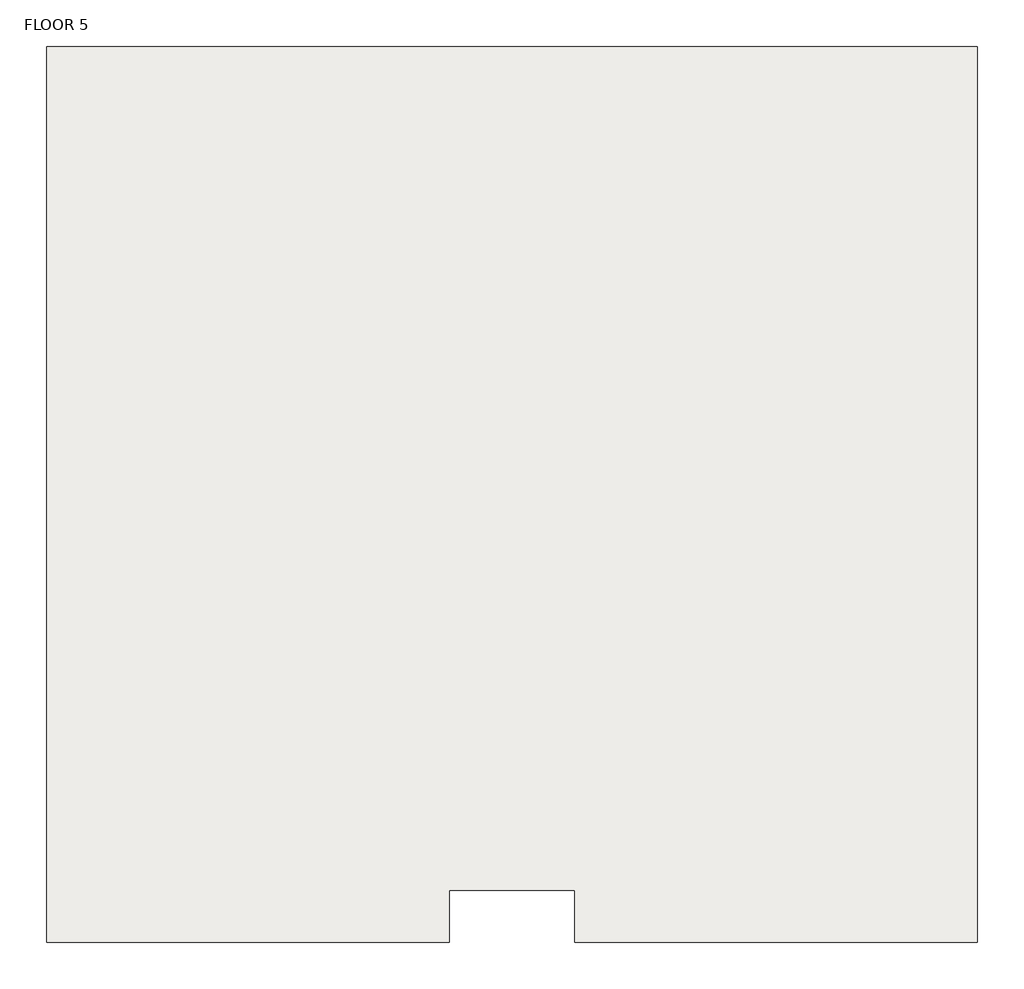
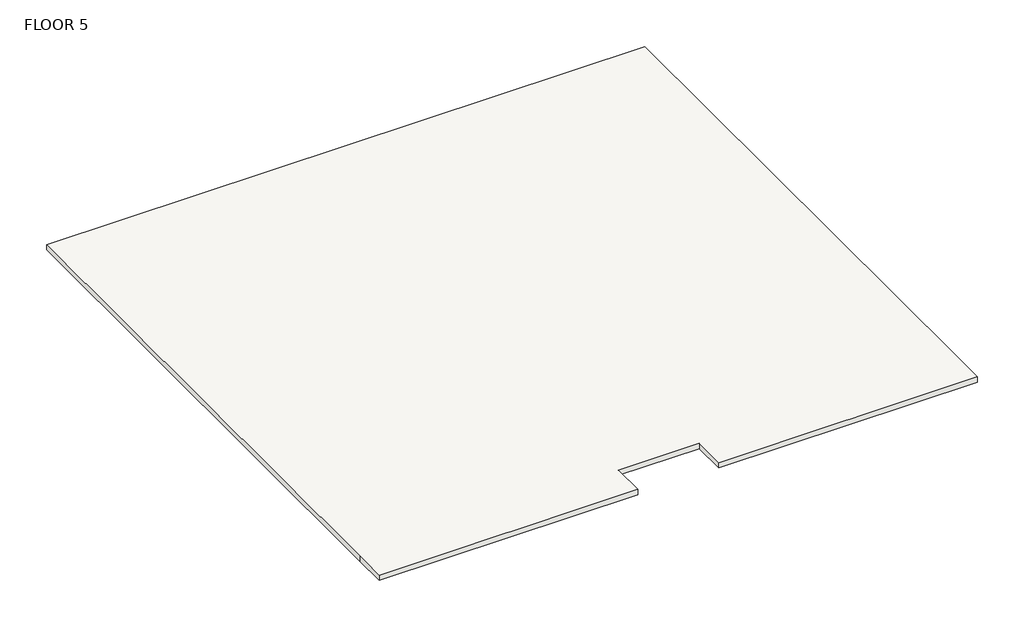
# One storey: 1 roof.
"""IFC4 building model written with IfcOpenShell, lengths in millimetres."""

from ifc_helpers import new_model, si_unit, frame, origin, place, context, project, spatial, polyline, outline, extrude, element, save

model = new_model("IFC4")

# Units and contexts
model_context = context("Model", 3, world=origin())
ifc_project = project(units=[si_unit("LENGTHUNIT", "METRE", prefix="MILLI")], contexts=[model_context])

# Site, building, storey
site = spatial("IfcSite", under=ifc_project)
building = spatial("IfcBuilding", under=site)
storey = spatial("IfcBuildingStorey", under=building, Name="FLOOR 5", Elevation=9391.9725604)

# Roof
placement = place(None, origin())
element("IfcRoof", 1, ObjectType="ROOFING 6\"", at=placement, inside=storey, context=model_context, shape_type="SweptSolid", body=[
    extrude(outline(polyline([(-3159.4137331, -7822.4593836), (-5369.2137331, -7822.4593836), (-5369.2137331, -8736.8593836), (-12430.4137331, -8736.8593836), (-12430.4137331, -7822.4593836), (-12430.4137331, 6987.3281164), (3901.7862669, 6987.3281164), (3901.7862669, -7822.4593836), (3901.7862669, -8736.8593836), (-3159.4137331, -8736.8593836), (-3159.4137331, -7822.4593836)])), frame((0.0, 0.0, 9391.9725604), z_axis=(0.0, 0.0, 1.0), x_axis=(1.0, 0.0, 0.0)), (0.0, 0.0, 1.0), 152.4),
])

save(model, "model.ifc")

# Revit data of these elements
# Type "ROOFING 6\""
#   Assembly Code = "B1020"
#   Layers, outside or top first: 0' - 6" no material (function 1)
# Element 1 (IfcRoof, "ROOFING 6\"")
#   built-in parameter 1001705 = 31.3136 (stored number, unit not read)
#   built-in parameter 1001710 = 33615
#   Phase Created = New Construction
#   Materials on its faces: "Default Roof"
# Materials
#   "Default Roof": colour RGB 88 101 114, transparency 0, Cost = 0
